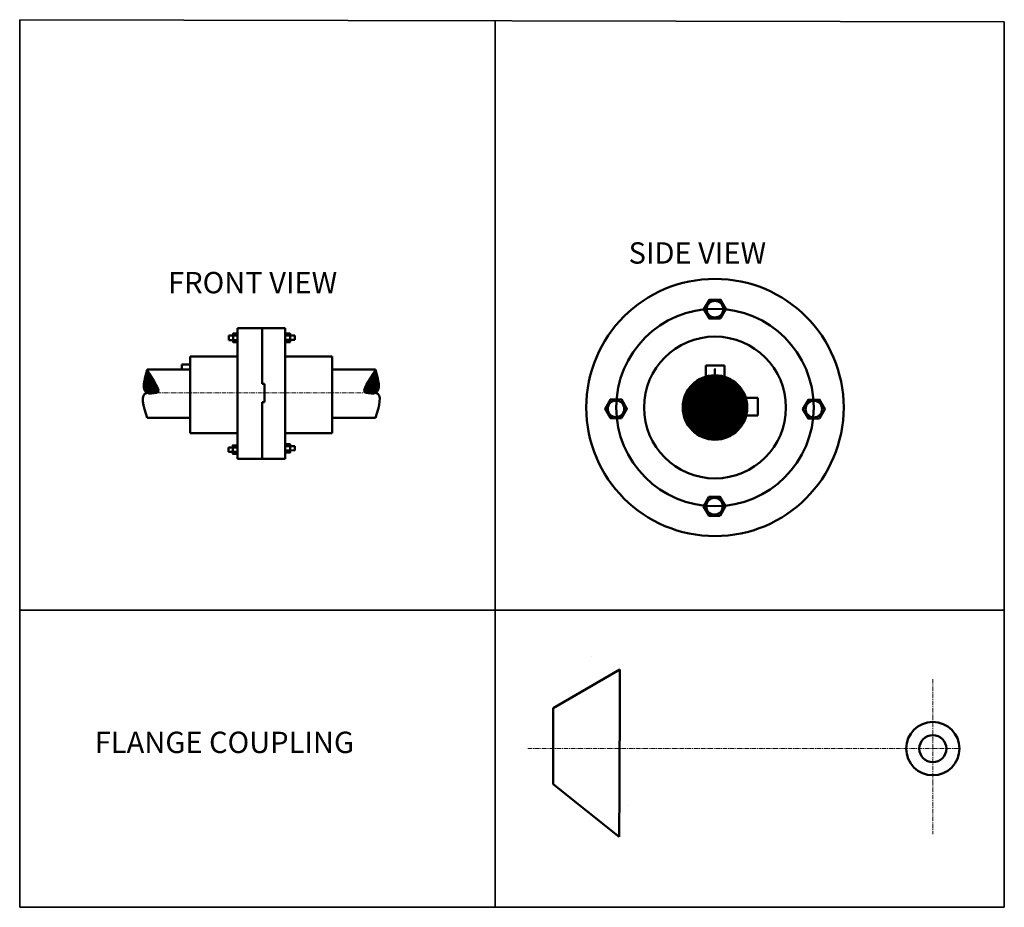
# Model space of a CAD drawing. Units: millimetres. Extents: x -29 to 6895, y -2105 to 4140.
import ezdxf

# ---------------------------------------------------------------- set-up
doc = ezdxf.new("R2010")
doc.units = ezdxf.units.MM
doc.linetypes.add('CENTER', pattern=[50.800000000000004, 31.75, -6.349999999999999, 6.349999999999999, -6.349999999999999])
for name, color, linetype, lineweight in [('M-CNTR', 1, 'CENTER', 18), ('M-HATC', 8, 'Continuous', 18), ('M-OUTL', 7, 'Continuous', 50), ('M-TEXT', 3, 'Continuous', 25), ('M-TTLB', 7, 'Continuous', 35)]:
    doc.layers.add(name, color=color, linetype=linetype, lineweight=lineweight)
doc.styles.get("Standard").update_dxf_attribs({"font": 'arial.ttf'})
pattern_1 = [(45, (491.5224746779131, -42.10088584851109), (-2.245064030267288, 2.245064030267288), [])]

# ---------------------------------------------------------------- blocks, each defined once
blk = doc.blocks.new('BOLT-HEAD-SIDE')
for p, q in [((1471.471257492727, 1917.734561807943), (1442.620241996361, 1917.734561807943)), ((1442.620241996361, 1917.734561807943), (1442.620241996361, 1885.544992205549)), ((1471.471257492727, 1885.544992205549), (1442.620241996361, 1885.544992205549)), ((1471.471257492727, 1917.734561807943), (1503.432144215383, 1917.734561807943)), ((1471.471257492727, 1885.544992205549), (1503.432144215383, 1885.544992205549))]:
    blk.add_line(p, q)
blk.add_lwpolyline([(1503.432144215383, 1931.266912811005), (1471.471257492727, 1931.266912811005), (1471.471257492727, 1872.585292868713), (1503.432144215383, 1872.585292868713)])
blk = doc.blocks.new('BOLT-NUT-SIDE')
for p, q in [((1872.900472306906, 1917.60221594975), (1837.328632342, 1917.515885326767)), ((1872.900472306906, 1888.576730322452), (1837.328632342, 1888.48867794269)), ((1872.900472306906, 1917.60221594975), (1905.251762989021, 1917.481852220092)), ((1905.242727002397, 1888.456400211392), (1872.900472306906, 1888.576730322452)), ((1905.251762989021, 1917.481852220092), (1905.242727002397, 1888.456400211392))]:
    blk.add_line(p, q)
blk.add_lwpolyline([(1837.328632342, 1931.266912811005), (1872.900472306906, 1931.266912811005), (1872.900472306906, 1872.585292868713), (1837.328632342, 1872.585292868713)], close=True)
blk = doc.blocks.new('BOLT-NUT-END')
blk.add_lwpolyline([(4898.892180909837, 2037.528796529043), (4936.815926198523, 2104.259652044876), (4897.987182749885, 2170.468006629444), (4821.234694012563, 2169.94550569818), (4783.310948723877, 2103.214650182347), (4822.139692172514, 2037.006295597779)], close=True)
blk.add_circle((4860.063437461199, 2103.737151113611), 58.3368524967283)

msp = doc.modelspace()

# ---------------------------------------------------------------- hatches: boundary and pattern name
at = {"layer": 'M-HATC'}
h = msp.add_hatch(dxfattribs=at)
h.set_pattern_fill('ANSI31', color=256)
h.set_pattern_definition(pattern_1)
edge = h.paths.add_edge_path()
edge.add_spline(control_points=[(934.9438962619859, 1515.164892118195), (934.9438962631477, 1515.16489211846), (975.5872897041536, 1524.458597022831), (902.9768510712017, 1607.982329871664), (867.6138232065151, 1679.245969113759)], knot_values=[243.1497986124911, 243.1497986124911, 243.1497986124911, 243.1497986124911, 243.149798617561, 420.5080196446312, 420.5080196446312, 420.5080196446312, 420.5080196446312], degree=3, periodic=0)
edge.add_spline(control_points=[(867.6138232065151, 1679.245969113759), (847.477909051215, 1605.994324252711), (819.0864852585818, 1502.710287743741), (910.9063361390243, 1510.109769854693), (934.943896265779, 1515.164892118992)], knot_values=[0, 0, 0, 0, 164.0810874520296, 231.3525799860705, 231.3525799860705, 231.3525799860705, 231.3525799860705], degree=3, periodic=0)
h = msp.add_hatch(dxfattribs=at)
h.set_pattern_fill('ANSI31', color=256)
h.set_pattern_definition(pattern_1)
edge = h.paths.add_edge_path()
edge.add_spline(control_points=[(2473.088372825644, 1515.164892118992), (2513.418781661468, 1532.742679391663), (2493.282867506168, 1605.994324252711), (2473.146953350868, 1679.245969113759)], knot_values=[0, 0, 0, 9.095e-13, 164.0810874520306, 164.0810874520306, 164.0810874520306, 164.0810874520306], degree=3, periodic=0)
edge.add_spline(control_points=[(2473.146953350868, 1679.245969113759), (2437.783925486181, 1607.982329871664), (2365.17348685323, 1524.458597022832), (2405.816880294235, 1515.164892118461), (2405.816880295397, 1515.164892118195)], knot_values=[243.149798612491, 243.149798612491, 243.149798612491, 243.149798612491, 420.5080196395612, 420.5080196446311, 420.5080196446311, 420.5080196446311, 420.5080196446311], degree=3, periodic=0)
edge.add_line((2405.81688029375, 1515.164892118992), (2473.088372825644, 1515.164892118992))
h = msp.add_hatch(dxfattribs=at)
h.set_pattern_fill('ANSI31', color=256)
h.set_pattern_definition([(45, (130.8984358907328, -145.4133447038093), (-2.245064030267288, 2.245064030267288), [])])
h.paths.add_polyline_path([(4860.672723351204, 1638.542745379921, 0.4142135623730977), (4633.982411234984, 1411.852433263697), (4860.672723351204, 1411.852433263698)])
h.paths.add_polyline_path([(5087.363035467426, 1411.852433263699), (4860.672723351204, 1411.852433263698), (4860.672723351204, 1185.162121147477, 0.4142135623730942)])
h.paths.add_polyline_path([(4860.672723351204, 1638.542745379921), (4860.672723351204, 1411.852433263698), (5087.363035467426, 1411.852433263699, 0.414213562373096)])
h.paths.add_polyline_path([(4860.672723351204, 1411.852433263698), (4633.982411234984, 1411.852433263697, 0.4142135623730925), (4860.672723351204, 1185.162121147477)])

# ---------------------------------------------------------------- linework, layer by layer
at = {"layer": 'M-CNTR'}
for p, q in [((934.9438962657758, 1515.164892118992), (1837.328632342, 1515.164892118991)), ((2473.088372825612, 1515.164892118992), (1837.328632341999, 1515.164892118991)), ((6392.707687830669, -499.3988497445243), (6392.707687830669, -1590.455182256934)), ((3543.729571677162, -988.1010747778345), (6580.365849729743, -988.1010747778345))]:
    msp.add_line(p, q, dxfattribs=at)
at = {"layer": 'M-OUTL'}
for p, q in [((1503.432144215383, 1971.064285573407), (1503.432144215383, 1050.445468117431)), ((1503.432144215383, 1971.064285573407), (1837.328632342, 1971.064285573407)), ((1676.563657110748, 1971.064285573407), (1676.563657110748, 1578.302825976482)), ((1837.328632342, 1971.064285573407), (1837.328632342, 1050.445468117431)), ((1422.508291576254, 1769.712231840349), (1171.035676039495, 1769.712231840349)), ((1171.035676039495, 1769.712231840349), (1171.035676039495, 1232.07965936627)), ((1422.508291576254, 1769.712231840349), (1503.432144215383, 1769.712231840349)), ((1837.328632342, 1769.712231840349), (1837.328632342, 1232.07965936627)), ((1918.252484981128, 1769.712231840349), (1837.328632341999, 1769.712231840349)), ((1918.252484981128, 1769.712231840349), (2169.725100517887, 1769.712231840349)), ((2169.725100517887, 1769.712231840349), (2169.725100517888, 1232.07965936627)), ((1072.135218033592, 1679.245969113759), (867.6138232065151, 1679.245969113759)), ((1072.135218033592, 1679.245969113759), (1171.035676039495, 1679.245969113759)), ((1171.035676039495, 1714.447905240774), (1111.210657097641, 1714.447905240774)), ((1111.210657097641, 1714.447905240774), (1111.210657097641, 1679.245969113759)), ((2268.62555852379, 1679.245969113759), (2169.725100517887, 1679.245969113759)), ((2268.62555852379, 1679.245969113759), (2473.146953350868, 1679.245969113759)), ((4795.524226469725, 1707.364266788283), (4928.171561616613, 1707.364266788283)), ((4795.524226469725, 1707.364266788283), (4795.524226469725, 1628.979518081402)), ((4928.171561616613, 1707.364266788283), (4928.171561616613, 1707.364266788283)), ((4928.171561616613, 1707.364266788283), (4928.171561616613, 1707.364266788283)), ((4928.171561616613, 1707.364266788283), (4928.171561616613, 1628.260391620527)), ((1676.563657110748, 1578.302825976482), (1693.306885216012, 1578.302825976482)), ((1693.306885216012, 1578.302825976482), (1693.306885216012, 1449.495618099732)), ((5076.816476836202, 1480.192578396459), (5163.242224038049, 1480.192578396459)), ((5163.242224038049, 1480.192578396459), (5163.242224038049, 1355.351975051794)), ((1693.306885216012, 1449.495618099732), (1676.563657110748, 1449.495618099732)), ((1676.563657110748, 1449.495618099732), (1676.563657110748, 1050.445468117431)), ((867.7351961212617, 1339.286597244258), (1171.035676039495, 1339.286597244258)), ((2473.025580436122, 1339.286597244258), (2169.725100517888, 1339.286597244258)), ((5163.242224038049, 1355.351975051794), (5080.20904341965, 1355.351975051794)), ((1171.035676039495, 1232.07965936627), (1503.432144215383, 1232.07965936627)), ((2169.725100517888, 1232.07965936627), (1837.328632342, 1232.079659366269)), ((1837.328632342, 1050.445468117431), (1503.432144215383, 1050.445468117431)), ((3992.805753136054, -339.6862145501071), (3992.805753136054, -339.6862145501071)), ((3722.615559363272, -704.2808767722454), (4192.704219248145, -431.7496609820518)), ((4192.704219248145, -431.7496609820518), (4192.704219248262, -593.1168392977561)), ((4192.704219248262, -593.1168392977561), (4188.592331073439, -1271.117925044824)), ((3722.615559363272, -704.2808767722454), (3722.615559363272, -1052.117505020753)), ((3722.615559363272, -1052.117505020753), (3722.615559363272, -1238.586674474936)), ((3722.615559363272, -1238.586674474936), (4186.548908467692, -1608.053825641546)), ((4186.548908467692, -1608.053825641546), (4188.592331073439, -1271.117925044824)), ((4242.942822367186, -1385.610178401286), (4242.942822367186, -1385.610178401286))]:
    msp.add_line(p, q, dxfattribs=at)
for points in [[(4860.672723351204, 1910.785403736358), (4860.672723351204, 1910.785403736358), (4860.672723351204, 1910.785403736358), (4860.672723351204, 1910.785403736358)], [(4860.672723351204, 1638.542745379921), (4860.672723351204, 1638.542745379921), (4860.672723351204, 1681.776410451753), (4860.672723351204, 1681.776410451753)], [(4860.672723351204, 1638.542745379921), (4860.672723351204, 1638.542745379921), (4860.672723351204, 1638.542745379921), (4860.672723351204, 1638.542745379921)], [(4860.672723351204, 1638.542745379921), (4860.672723351204, 1638.542745379921), (4860.672723351204, 1638.542745379921), (4860.672723351204, 1638.542745379921)], [(4860.672723351204, 1638.542745379921), (4860.672723351204, 1638.542745379921), (4860.672723351204, 1638.542745379921), (4860.672723351204, 1638.542745379921)], [(4860.672723351204, 1638.542745379921), (4860.672723351204, 1638.542745379921), (4860.672723351204, 1411.852433263699), (4860.672723351204, 1411.852433263699)], [(4860.672723351204, 1638.542745379921), (4860.672723351204, 1638.542745379921), (4860.672723351204, 1638.542745379921), (4860.672723351204, 1638.542745379921)]]:
    msp.add_lwpolyline(points, close=True, dxfattribs=at)
for centre, radius in [((4860.672723351204, 1411.852433263699), 905.0520640186915), ((4860.672723351204, 1411.852433263699), 694.7579918853886), ((4860.672723351204, 1411.852433263699), 498.9329704726586), ((4860.672723351204, 1411.852433263699), 226.6903121162218), ((6392.707687830669, -988.1010747778345), 187.6581618990749), ((6392.707687830669, -988.1010747778345), 95.35230619841462)]:
    msp.add_circle(centre, radius, dxfattribs=at)
for points, knots in [([(867.6138232065151, 1679.245969113759), (847.477909051215, 1605.994324252711), (819.0864852585818, 1502.710287743741), (910.9063361390243, 1510.109769854693), (934.943896265779, 1515.164892118992)], [0, 0, 0, 0, 164.0810874520296, 231.3525799860705, 231.3525799860705, 231.3525799860705, 231.3525799860705]), ([(934.9438962619859, 1515.164892118195), (934.9438962631477, 1515.16489211846), (975.5872897041536, 1524.458597022831), (902.9768510712017, 1607.982329871664), (867.6138232065151, 1679.245969113759)], [243.1497986124911, 243.1497986124911, 243.1497986124911, 243.1497986124911, 243.149798617561, 420.5080196446312, 420.5080196446312, 420.5080196446312, 420.5080196446312]), ([(2405.816880295397, 1515.164892118195), (2405.816880294235, 1515.164892118461), (2365.17348685323, 1524.458597022832), (2437.783925486181, 1607.982329871664), (2473.146953350868, 1679.245969113759)], [243.1497986124911, 243.1497986124911, 243.1497986124911, 243.1497986124911, 243.149798617561, 420.5080196446312, 420.5080196446312, 420.5080196446312, 420.5080196446312]), ([(2473.146953350868, 1679.245969113759), (2493.282867506168, 1605.994324252711), (2521.674291298801, 1502.710287743742), (2429.854440418359, 1510.109769854693), (2405.816880291604, 1515.164892118993)], [0, 0, 0, 0, 164.0810874520296, 231.3525799860705, 231.3525799860705, 231.3525799860705, 231.3525799860705])]:
    msp.add_open_spline(points, degree=3, knots=knots, dxfattribs=at)
for points in [[(867.7351961212617, 1339.286597244258), (841.3681182600434, 1422.481743429637), (815.0010403988254, 1505.676889615015), (867.6724037317704, 1515.164892118992)], [(2473.025580436122, 1339.286597244258), (2499.39265829734, 1422.481743429637), (2525.759736158557, 1505.676889615015), (2473.088372825613, 1515.164892118992)]]:
    msp.add_open_spline(points, degree=3, dxfattribs=at)
at = {"layer": 'M-TTLB'}
for p, q in [((-28.63075130328798, 2544.00310804143), (-28.63075130328798, 4140.297417892281)), ((-28.63075130328798, 4140.297417892281), (6895.310250567877, 4126.263805723222)), ((3314.21798459784, 4133.522050700851), (3314.217984597839, -2104.664816342301)), ((6895.310250567876, 4126.263805723222), (6895.310250567876, -2104.664816342301)), ((-28.63075130328798, 2544.00310804143), (-28.63075130328799, -2104.664816342302)), ((-28.63075130328798, -13.65499133569756), (6895.310250567877, -13.65499133569756)), ((-28.63075130328798, -2104.664816342301), (6895.310250567876, -2104.664816342301))]:
    msp.add_line(p, q, dxfattribs=at)

# ---------------------------------------------------------------- block references
at = {"layer": 'M-OUTL'}
for name, p in [('BOLT-NUT-END', (0, 0)), ('BOLT-HEAD-SIDE', (0, 0)), ('BOLT-NUT-SIDE', (0, 0)), ('BOLT-NUT-END', (-695.445281064719, -701.1558820545746)), ('BOLT-NUT-END', (696.0707685822035, -703.2723812033786)), ('BOLT-HEAD-SIDE', (-2.027774876981766, -786.1910387238753)), ('BOLT-NUT-SIDE', (-6.8212e-12, -778.0859771370455)), ('BOLT-NUT-END', (-2.86424180974609, -1386.900381601606))]:
    msp.add_blockref(name, p, dxfattribs=at)

# ---------------------------------------------------------------- texts
at = {"layer": 'M-TEXT', "char_height": 150, "attachment_point": 1}
for s, insert in [('SIDE VIEW', (4253.243509778513, 2574.033064758895)), ('FRONT VIEW', (1015.159879823084, 2365.279068926822)), ('FLANGE COUPLING', (499.1326276628533, -869.1318794835241))]:
    msp.add_mtext(s, dxfattribs=dict(at, insert=insert))

doc.saveas('drawing.dxf')
